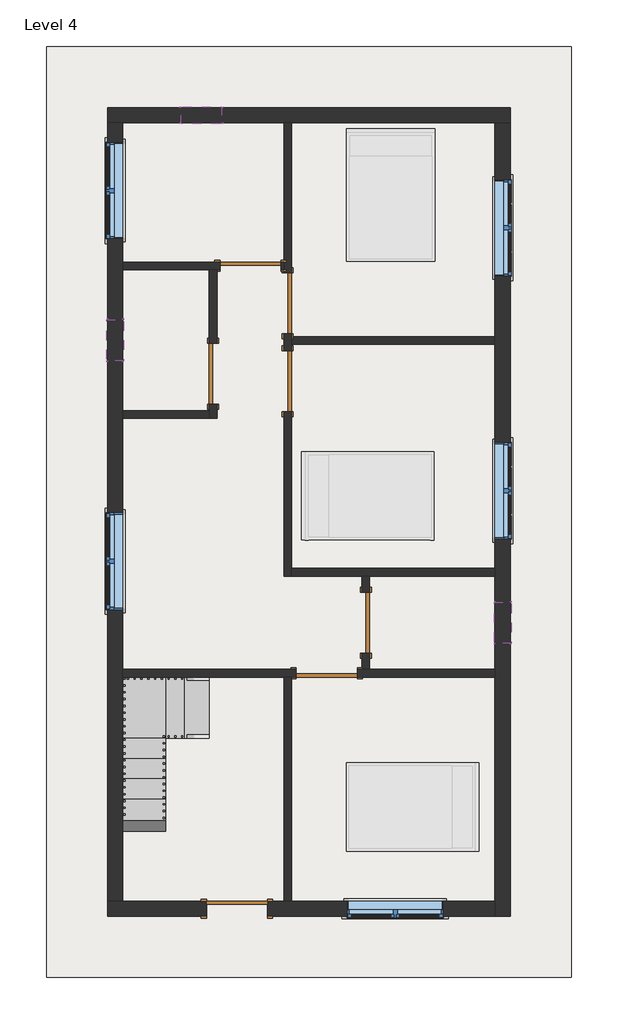
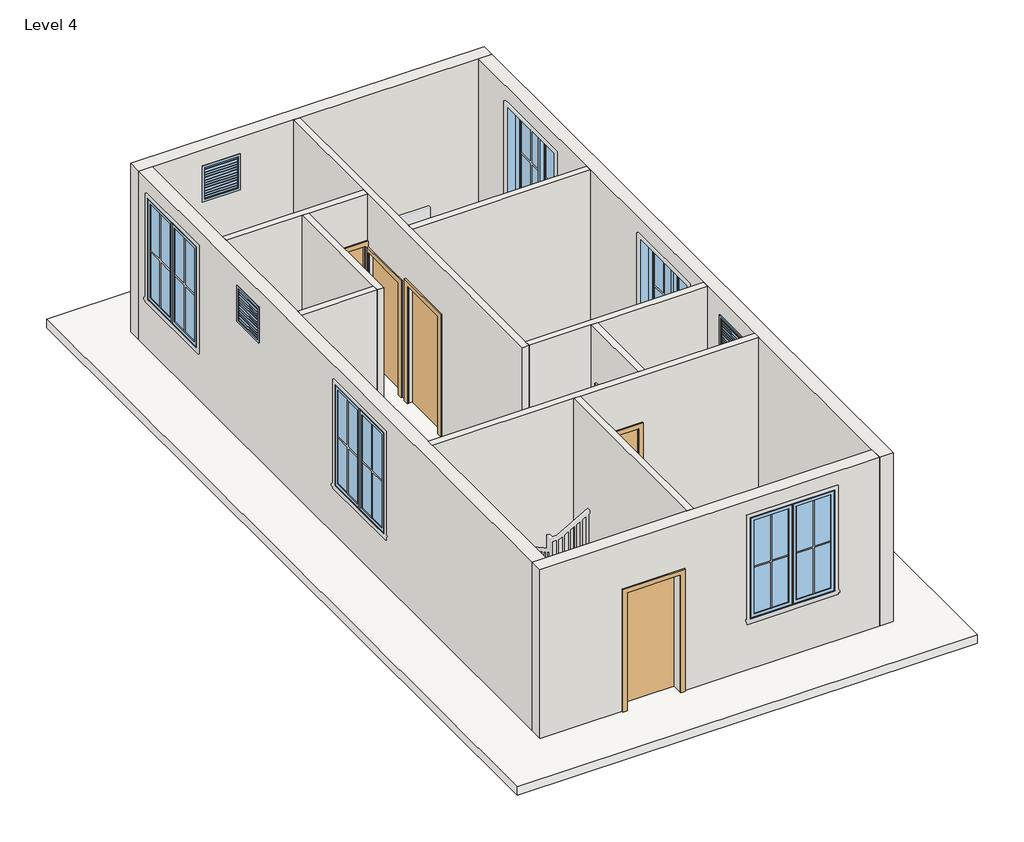
# One storey, part 1 of 2: 13 walls, 8 windows, 7 doors, 1 roof, 1 stair flight.
"""IFC4 building model written with IfcOpenShell, lengths in millimetres."""

from ifc_helpers import new_model, si_unit, frame, origin, place, context, project, spatial, polyline, outline, extrude, faceted_brep, transform, mapped, element, save
from components import door_5e62189b, door_17d80c48, door_e5f9f3c4, door_305aa2a5, door_0ca8825f, window_9ac97e1a, window_f2d8fef0

model = new_model("IFC4")

# Units and contexts
model_context = context("Model", 3, world=origin())
ifc_project = project(units=[si_unit("LENGTHUNIT", "METRE", prefix="MILLI")], contexts=[model_context])

# Site, building, storey
site = spatial("IfcSite", under=ifc_project)
building = spatial("IfcBuilding", under=site)
storey = spatial("IfcBuildingStorey", under=building, Name="Level 4", Elevation=6400.8)

# Doors
placement = place(None, origin())
door_shape = door_5e62189b(model_context)
element("IfcDoor", 1, ObjectType="Single-Flush : 36\" x 80\"", at=placement, inside=storey, context=model_context, shape_type="MappedRepresentation", body=[
    mapped(door_shape, transform((-2690.3389285, 2204.6069249, 6400.8), x_axis=(0.0, -1.0, 0.0), y_axis=(1.0, 0.0, 0.0), z_axis=(0.0, 0.0, 1.0))),
])
element("IfcDoor", 2, ObjectType="Single-Flush : 36\" x 80\"", at=placement, inside=storey, context=model_context, shape_type="MappedRepresentation", body=[
    mapped(door_shape, transform((-404.3389285, -1522.8430751, 6400.8), x_axis=(0.0, 1.0, 0.0), y_axis=(-1.0, 0.0, 0.0), z_axis=(0.0, 0.0, 1.0))),
])
door_2_shape = door_17d80c48(model_context)
element("IfcDoor", 3, ObjectType="Single-Flush : 36\" x 80\"", at=placement, inside=storey, context=model_context, shape_type="MappedRepresentation", body=[
    mapped(door_2_shape, transform((-1572.7389285, 3258.7069249, 6400.8), x_axis=(0.0, -1.0, 0.0), y_axis=(1.0, 0.0, 0.0), z_axis=(0.0, 0.0, 1.0))),
])
door_3_shape = door_e5f9f3c4(model_context)
element("IfcDoor", 4, ObjectType="Single-Flush : 36\" x 84\"", at=placement, inside=storey, context=model_context, shape_type="MappedRepresentation", body=[
    mapped(door_3_shape, transform((-2131.5389285, 3817.5069249, 6400.8), x_axis=(1.0, 0.0, 0.0), y_axis=(0.0, 1.0, 0.0), z_axis=(0.0, 0.0, 1.0))),
])
element("IfcDoor", 5, ObjectType="Single-Flush : 36\" x 84\"", at=placement, inside=storey, context=model_context, shape_type="MappedRepresentation", body=[
    mapped(door_3_shape, transform((-988.5389285, -2278.4930751, 6400.8), x_axis=(-1.0, 0.0, 0.0), y_axis=(0.0, -1.0, 0.0), z_axis=(0.0, 0.0, 1.0))),
])
door_4_shape = door_305aa2a5(model_context)
element("IfcDoor", 6, ObjectType="Single-Flush : 36\" x 84\"", at=placement, inside=storey, context=model_context, shape_type="MappedRepresentation", body=[
    mapped(door_4_shape, transform((-1572.7389285, 2090.3069249, 6400.8), x_axis=(0.0, 1.0, 0.0), y_axis=(-1.0, 0.0, 0.0), z_axis=(0.0, 0.0, 1.0))),
])
door_5_shape = door_0ca8825f(model_context)
element("IfcDoor", 7, ObjectType="Single-Flush : 36\" x 84\"", at=placement, inside=storey, context=model_context, shape_type="MappedRepresentation", body=[
    mapped(door_5_shape, transform((-2334.7389285, -5802.7430751, 6400.8), x_axis=(1.0, 0.0, 0.0), y_axis=(0.0, 1.0, 0.0), z_axis=(0.0, 0.0, 1.0))),
])

# Roof
element("IfcRoof", 8, ObjectType="ROOF 6\"", at=placement, inside=storey, context=model_context, shape_type="SweptSolid", body=[
    extrude(outline(polyline([(-5185.8889285, 7100.4569249), (2675.4110715, 7100.4569249), (2675.4110715, -6831.4430751), (-5185.8889285, -6831.4430751), (-5185.8889285, 7100.4569249)])), frame((0.0, 0.0, 6248.4), z_axis=(0.0, 0.0, 1.0), x_axis=(1.0, 0.0, 0.0)), (0.0, 0.0, 1.0), 152.4),
])

# Stair flight
element("IfcStairFlight", 9, ObjectType="3/4\" Nosing", at=placement, inside=storey, context=model_context, shape_type="Brep", body=[
    faceted_brep([(-2747.4889285, -3250.0430751, 6570.1333333), (-2747.4889285, -2335.6430751, 6570.1333333), (-3128.4889285, -2335.6430751, 6570.1333333), (-3128.4889285, -3250.0430751, 6570.1333333), (-3128.4889285, -3250.0430751, 6506.6333333), (-2754.6326785, -3250.0430751, 6506.6333333), (-2754.6326785, -2335.6430751, 6506.6333333), (-3128.4889285, -2335.6430751, 6506.6333333)], [[[0, 1, 2, 3]], [[0, 3, 4, 5]], [[2, 1, 6, 7]], [[1, 0, 5, 6]], [[4, 7, 6, 5]], [[7, 4, 3, 2]]]),
    faceted_brep([(-3128.4889285, -3250.0430751, 6739.4666667), (-3128.4889285, -2335.6430751, 6739.4666667), (-3401.5389285, -2335.6430751, 6739.4666667), (-3401.5389285, -3250.0430751, 6739.4666667), (-3401.5389285, -3250.0430751, 6675.9666667), (-3135.6326785, -3250.0430751, 6675.9666667), (-3135.6326785, -2335.6430751, 6675.9666667), (-3401.5389285, -2335.6430751, 6675.9666667)], [[[0, 1, 2, 3]], [[0, 3, 4, 5]], [[2, 1, 6, 7]], [[1, 0, 5, 6]], [[4, 7, 6, 5]], [[7, 4, 3, 2]]]),
    faceted_brep([(-3401.5389285, -3269.0930751, 6908.8), (-3401.5389285, -3250.0430751, 6908.8), (-3401.5389285, -2335.6430751, 6908.8), (-4042.8889285, -2335.6430751, 6908.8), (-4042.8889285, -3269.0930751, 6908.8), (-3401.5389285, -3269.0930751, 6845.3), (-3401.5389285, -3250.0430751, 6845.3), (-3408.6826785, -3250.0430751, 6845.3), (-3408.6826785, -2335.6430751, 6845.3), (-4042.8889285, -2335.6430751, 6845.3), (-4042.8889285, -3269.0930751, 6845.3), (-3401.5389285, -3250.0430751, 7078.1333333), (-4042.8889285, -3250.0430751, 7078.1333333), (-4042.8889285, -3285.5502386, 7078.1333333), (-4042.8889285, -3573.8930751, 7078.1333333), (-3401.5389285, -3573.8930751, 7078.1333333), (-3401.5389285, -3285.5502386, 7078.1333333), (-3401.5389285, -3573.8930751, 7005.5200976), (-3401.5389285, -3285.5502386, 6845.3), (-4042.8889285, -3285.5502386, 6845.3), (-4042.8889285, -3573.8930751, 7005.5200976), (-3401.5389285, -3554.8430751, 7247.4666667), (-4042.8889285, -3554.8430751, 7247.4666667), (-4042.8889285, -3878.6930751, 7247.4666667), (-3401.5389285, -3878.6930751, 7247.4666667), (-3401.5389285, -3878.6930751, 7174.8847552), (-4042.8889285, -3878.6930751, 7174.8847552), (-3401.5389285, -3859.6430751, 7416.8), (-4042.8889285, -3859.6430751, 7416.8), (-4042.8889285, -4183.4930751, 7416.8), (-3401.5389285, -4183.4930751, 7416.8), (-3401.5389285, -4183.4930751, 7344.2494128), (-4042.8889285, -4183.4930751, 7344.2494128), (-3401.5389285, -4164.4430751, 7586.1333333), (-4042.8889285, -4164.4430751, 7586.1333333), (-4042.8889285, -4488.2930751, 7586.1333333), (-3401.5389285, -4488.2930751, 7586.1333333), (-3401.5389285, -4488.2930751, 7513.6140703), (-4042.8889285, -4488.2930751, 7513.6140703), (-3401.5389285, -4792.8112092, 7755.4666667), (-3401.5389285, -4469.2430751, 7755.4666667), (-4042.8889285, -4469.2430751, 7755.4666667), (-4042.8889285, -4792.8112092, 7755.4666667), (-3401.5389285, -4773.7612092, 7924.8), (-3401.5389285, -5114.0119996, 7924.8), (-3401.5389285, -5114.0119996, 7861.3), (-4042.8889285, -4792.8112092, 7682.8221068), (-4042.8889285, -4773.7612092, 7924.8), (-4042.8889285, -5114.0119996, 7924.8), (-4042.8889285, -5688.4430751, 7924.8), (-3401.5389285, -5688.4430751, 7924.8), (-4042.8889285, -5114.0119996, 7861.3), (-4042.8889285, -5688.4430751, 7861.3), (-3401.5389285, -5688.4430751, 7861.3)], [[[0, 1, 2, 3, 4]], [[1, 0, 5, 6]], [[7, 1, 6]], [[3, 2, 8, 9]], [[4, 3, 9, 10]], [[11, 12, 13, 14, 15, 16]], [[0, 11, 16, 15, 17, 18, 5]], [[12, 4, 10, 19, 20, 14, 13]], [[21, 22, 23, 24]], [[21, 24, 25, 17, 15]], [[23, 22, 14, 20, 26]], [[27, 28, 29, 30]], [[27, 30, 31, 25, 24]], [[29, 28, 23, 26, 32]], [[33, 34, 35, 36]], [[33, 36, 37, 31, 30]], [[35, 34, 29, 32, 38]], [[39, 40, 41, 42]], [[39, 43, 44, 45, 37, 36, 40]], [[42, 41, 35, 38, 46]], [[43, 47, 48, 49, 50, 44]], [[47, 42, 46, 51, 52, 49, 48]], [[50, 49, 52, 53]], [[2, 1, 7, 8]], [[0, 4, 12, 11]], [[15, 14, 22, 21]], [[24, 23, 28, 27]], [[30, 29, 34, 33]], [[36, 35, 41, 40]], [[39, 42, 47, 43]], [[18, 19, 10, 9, 8, 7, 6, 5]], [[19, 18, 17, 25, 31, 37, 45, 51, 46, 38, 32, 26, 20]], [[45, 53, 52, 51]], [[53, 45, 44, 50]]]),
    faceted_brep([(-3401.5389285, -4773.7612092, 8094.1333333), (-3401.5389285, -5688.4430751, 8094.1333333), (-3128.4889285, -5688.4430751, 8094.1333333), (-3128.4889285, -4773.7612092, 8094.1333333), (-3394.3951785, -4773.7612092, 8030.6333333), (-3128.4889285, -4773.7612092, 8030.6333333), (-3394.3951785, -5688.4430751, 8030.6333333), (-3128.4889285, -5688.4430751, 8030.6333333)], [[[0, 1, 2, 3]], [[4, 0, 3, 5]], [[2, 1, 6, 7]], [[1, 0, 4, 6]], [[5, 7, 6, 4]], [[7, 5, 3, 2]]]),
    faceted_brep([(-3128.4889285, -4773.7612092, 8263.4666667), (-3128.4889285, -5688.4430751, 8263.4666667), (-2793.6303845, -5688.4430751, 8263.4666667), (-2793.6303845, -4773.7612092, 8263.4666667), (-2793.6303845, -4773.7612092, 8199.9666667), (-3121.3451785, -4773.7612092, 8199.9666667), (-3121.3451785, -5688.4430751, 8199.9666667), (-2793.6303845, -5688.4430751, 8199.9666667)], [[[0, 1, 2, 3]], [[0, 3, 4, 5]], [[2, 1, 6, 7]], [[3, 2, 7, 4]], [[1, 0, 5, 6]], [[6, 5, 4, 7]]]),
])

# Walls
element("IfcWall", 10, ObjectType="WALL 4.5\"", at=placement, inside=storey, context=model_context, shape_type="Brep", body=[
    faceted_brep([(-1629.8889285, 2801.5069249, 8432.8), (-1629.8889285, 2801.5069249, 6400.8), (-1629.8889285, 2547.5069249, 6400.8), (-1629.8889285, 2547.5069249, 8534.4), (-1629.8889285, 1633.1069249, 8534.4), (-1629.8889285, 1633.1069249, 6400.8), (-1629.8889285, -824.3430751, 6400.8), (-1629.8889285, -824.3430751, 9448.8), (-1629.8889285, 3760.3569249, 9448.8), (-1629.8889285, 3874.6569249, 9448.8), (-1629.8889285, 5957.4569249, 9448.8), (-1629.8889285, 5957.4569249, 6400.8), (-1629.8889285, 3874.6569249, 6400.8), (-1629.8889285, 3760.3569249, 6400.8), (-1629.8889285, 3715.9069249, 6400.8), (-1629.8889285, 3715.9069249, 8432.8), (-1515.5889285, 2547.5069249, 6400.8), (-1515.5889285, 2642.7569249, 6400.8), (-1515.5889285, 2757.0569249, 6400.8), (-1515.5889285, 2801.5069249, 6400.8), (-1515.5889285, 2801.5069249, 8432.8), (-1515.5889285, 3715.9069249, 8432.8), (-1515.5889285, 3715.9069249, 6400.8), (-1515.5889285, 5957.4569249, 6400.8), (-1515.5889285, 5957.4569249, 9448.8), (-1515.5889285, 2757.0569249, 9448.8), (-1515.5889285, 2642.7569249, 9448.8), (-1515.5889285, -710.0430751, 9448.8), (-1515.5889285, -824.3430751, 9448.8), (-1515.5889285, -824.3430751, 6400.8), (-1515.5889285, -710.0430751, 6400.8), (-1515.5889285, 1633.1069249, 6400.8), (-1515.5889285, 1633.1069249, 8534.4), (-1515.5889285, 2547.5069249, 8534.4)], [[[0, 1, 2, 3, 4, 5, 6, 7, 8, 9, 10, 11, 12, 13, 14, 15]], [[16, 17, 18, 19, 20, 21, 22, 23, 24, 25, 26, 27, 28, 29, 30, 31, 32, 33]], [[31, 30, 29, 6, 5]], [[2, 1, 19, 18, 17, 16]], [[14, 13, 12, 11, 23, 22]], [[11, 10, 24, 23]], [[3, 2, 16, 33]], [[4, 3, 33, 32]], [[5, 4, 32, 31]], [[20, 19, 1, 0]], [[21, 20, 0, 15]], [[22, 21, 15, 14]], [[10, 9, 8, 7, 28, 27, 26, 25, 24]], [[7, 6, 29, 28]]]),
])
element("IfcWall", 11, ObjectType="WALL 4.5\"", at=placement, inside=storey, context=model_context, shape_type="Brep", body=[
    faceted_brep([(1532.4110715, -710.0430751, 6400.8), (-1515.5889285, -710.0430751, 6400.8), (-1515.5889285, -710.0430751, 9448.8), (1532.4110715, -710.0430751, 9448.8), (1532.4110715, -824.3430751, 6400.8), (1532.4110715, -824.3430751, 9448.8), (-347.1889285, -824.3430751, 9448.8), (-461.4889285, -824.3430751, 9448.8), (-1515.5889285, -824.3430751, 9448.8), (-1515.5889285, -824.3430751, 6400.8), (-461.4889285, -824.3430751, 6400.8), (-347.1889285, -824.3430751, 6400.8)], [[[0, 1, 2, 3]], [[4, 5, 6, 7, 8, 9, 10, 11]], [[1, 0, 4, 11, 10, 9]], [[0, 3, 5, 4]], [[3, 2, 8, 7, 6, 5]], [[2, 1, 9, 8]]]),
])
element("IfcWall", 12, ObjectType="WALL 4.5\"", at=placement, inside=storey, context=model_context, shape_type="SweptSolid", body=[
    extrude(outline(polyline([(-1515.5889285, 2757.0569249), (1532.4110715, 2757.0569249), (1532.4110715, 2642.7569249), (-1515.5889285, 2642.7569249), (-1515.5889285, 2757.0569249)])), frame((0.0, 0.0, 6400.8), z_axis=(0.0, 0.0, 1.0), x_axis=(1.0, 0.0, 0.0)), (0.0, 0.0, 1.0), 3048.0),
])
element("IfcWall", 13, ObjectType="WALL 4.5\"", at=placement, inside=storey, context=model_context, shape_type="Brep", body=[
    faceted_brep([(-1674.3389285, 3760.3569249, 8534.4), (-1674.3389285, 3760.3569249, 6400.8), (-1629.8889285, 3760.3569249, 6400.8), (-1629.8889285, 3760.3569249, 9448.8), (-2633.1889285, 3760.3569249, 9448.8), (-2747.4889285, 3760.3569249, 9448.8), (-4042.8889285, 3760.3569249, 9448.8), (-4042.8889285, 3760.3569249, 6400.8), (-2747.4889285, 3760.3569249, 6400.8), (-2633.1889285, 3760.3569249, 6400.8), (-2588.7389285, 3760.3569249, 6400.8), (-2588.7389285, 3760.3569249, 8534.4), (-1629.8889285, 3874.6569249, 6400.8), (-1674.3389285, 3874.6569249, 6400.8), (-1674.3389285, 3874.6569249, 8534.4), (-2588.7389285, 3874.6569249, 8534.4), (-2588.7389285, 3874.6569249, 6400.8), (-4042.8889285, 3874.6569249, 6400.8), (-4042.8889285, 3874.6569249, 9448.8), (-1629.8889285, 3874.6569249, 9448.8)], [[[0, 1, 2, 3, 4, 5, 6, 7, 8, 9, 10, 11]], [[12, 13, 14, 15, 16, 17, 18, 19]], [[2, 1, 13, 12]], [[10, 9, 8, 7, 17, 16]], [[7, 6, 18, 17]], [[3, 2, 12, 19]], [[14, 13, 1, 0]], [[15, 14, 0, 11]], [[16, 15, 11, 10]], [[6, 5, 4, 3, 19, 18]]]),
])
element("IfcWall", 14, ObjectType="WALL 4.5\"", at=placement, inside=storey, context=model_context, shape_type="Brep", body=[
    faceted_brep([(-2747.4889285, 1747.4069249, 8432.8), (-2747.4889285, 1747.4069249, 6400.8), (-2747.4889285, 1652.1569249, 6400.8), (-2747.4889285, 1537.8569249, 6400.8), (-2747.4889285, 1537.8569249, 9448.8), (-2747.4889285, 1652.1569249, 9448.8), (-2747.4889285, 3760.3569249, 9448.8), (-2747.4889285, 3760.3569249, 6400.8), (-2747.4889285, 2661.8069249, 6400.8), (-2747.4889285, 2661.8069249, 8432.8), (-2633.1889285, 1537.8569249, 6400.8), (-2633.1889285, 1747.4069249, 6400.8), (-2633.1889285, 1747.4069249, 8432.8), (-2633.1889285, 2661.8069249, 8432.8), (-2633.1889285, 2661.8069249, 6400.8), (-2633.1889285, 3760.3569249, 6400.8), (-2633.1889285, 3760.3569249, 9448.8), (-2633.1889285, 1537.8569249, 9448.8)], [[[0, 1, 2, 3, 4, 5, 6, 7, 8, 9]], [[10, 11, 12, 13, 14, 15, 16, 17]], [[8, 7, 15, 14]], [[3, 2, 1, 11, 10]], [[7, 6, 16, 15]], [[4, 3, 10, 17]], [[12, 11, 1, 0]], [[13, 12, 0, 9]], [[14, 13, 9, 8]], [[6, 5, 4, 17, 16]]]),
])
element("IfcWall", 15, ObjectType="WALL 4.5\"", at=placement, inside=storey, context=model_context, shape_type="SweptSolid", body=[
    extrude(outline(polyline([(-4042.8889285, 1652.1569249), (-2747.4889285, 1652.1569249), (-2747.4889285, 1537.8569249), (-4042.8889285, 1537.8569249), (-4042.8889285, 1652.1569249)])), frame((0.0, 0.0, 6400.8), z_axis=(0.0, 0.0, 1.0), x_axis=(1.0, 0.0, 0.0)), (0.0, 0.0, 1.0), 3048.0),
])
element("IfcWall", 16, ObjectType="WALL 4.5\"", at=placement, inside=storey, context=model_context, shape_type="Brep", body=[
    faceted_brep([(-4042.8889285, -2335.6430751, 6400.8), (-1629.8889285, -2335.6430751, 6400.8), (-1515.5889285, -2335.6430751, 6400.8), (-1445.7389285, -2335.6430751, 6400.8), (-1445.7389285, -2335.6430751, 8534.4), (-531.3389285, -2335.6430751, 8534.4), (-531.3389285, -2335.6430751, 6400.8), (1532.4110715, -2335.6430751, 6400.8), (1532.4110715, -2335.6430751, 9448.8), (-1515.5889285, -2335.6430751, 9448.8), (-1629.8889285, -2335.6430751, 9448.8), (-4042.8889285, -2335.6430751, 9448.8), (-1445.7389285, -2221.3430751, 8534.4), (-1445.7389285, -2221.3430751, 6400.8), (-4042.8889285, -2221.3430751, 6400.8), (-4042.8889285, -2221.3430751, 9448.8), (-461.4889285, -2221.3430751, 9448.8), (-347.1889285, -2221.3430751, 9448.8), (1532.4110715, -2221.3430751, 9448.8), (1532.4110715, -2221.3430751, 6400.8), (-347.1889285, -2221.3430751, 6400.8), (-461.4889285, -2221.3430751, 6400.8), (-531.3389285, -2221.3430751, 6400.8), (-531.3389285, -2221.3430751, 8534.4)], [[[0, 1, 2, 3, 4, 5, 6, 7, 8, 9, 10, 11]], [[12, 13, 14, 15, 16, 17, 18, 19, 20, 21, 22, 23]], [[14, 13, 3, 2, 1, 0]], [[22, 21, 20, 19, 7, 6]], [[8, 7, 19, 18]], [[0, 11, 15, 14]], [[4, 3, 13, 12]], [[5, 4, 12, 23]], [[6, 5, 23, 22]], [[11, 10, 9, 8, 18, 17, 16, 15]]]),
])
element("IfcWall", 17, ObjectType="WALL 4.5\"", at=placement, inside=storey, context=model_context, shape_type="SweptSolid", body=[
    extrude(outline(polyline([(-824.3430751, 6400.8), (-1065.6430751, 6400.8), (-1065.6430751, 8432.8), (-1980.0430751, 8432.8), (-1980.0430751, 6400.8), (-2221.3430751, 6400.8), (-2221.3430751, 9448.8), (-824.3430751, 9448.8), (-824.3430751, 6400.8)])), frame((-461.4889285, 0.0, 0.0), z_axis=(1.0, 0.0, 0.0), x_axis=(0.0, 1.0, 0.0)), (0.0, 0.0, 1.0), 114.3),
])
element("IfcWall", 18, ObjectType="WALL 4.5\"", at=placement, inside=storey, context=model_context, shape_type="SweptSolid", body=[
    extrude(outline(polyline([(-1629.8889285, -5688.4430751), (-1629.8889285, -2335.6430751), (-1515.5889285, -2335.6430751), (-1515.5889285, -5688.4430751), (-1629.8889285, -5688.4430751)])), frame((0.0, 0.0, 6400.8), z_axis=(0.0, 0.0, 1.0), x_axis=(1.0, 0.0, 0.0)), (0.0, 0.0, 1.0), 3048.0),
])
element("IfcWall", 19, ObjectType="WALL 9\"", at=placement, inside=storey, context=model_context, shape_type="Brep", body=[
    faceted_brep([(-4271.4889285, 5957.4569249, 6400.8), (-4042.8889285, 5957.4569249, 6400.8), (-1629.8889285, 5957.4569249, 6400.8), (-1515.5889285, 5957.4569249, 6400.8), (1532.4110715, 5957.4569249, 6400.8), (1761.0110715, 5957.4569249, 6400.8), (1761.0110715, 5957.4569249, 9448.8), (1532.4110715, 5957.4569249, 9448.8), (-1515.5889285, 5957.4569249, 9448.8), (-1629.8889285, 5957.4569249, 9448.8), (-4042.8889285, 5957.4569249, 9448.8), (-4271.4889285, 5957.4569249, 9448.8), (-2560.1639285, 5957.4569249, 9144.0), (-2560.1639285, 5957.4569249, 8534.4), (-3169.7639285, 5957.4569249, 8534.4), (-3169.7639285, 5957.4569249, 9144.0), (-4271.4889285, 6186.0569249, 6400.8), (-4271.4889285, 6186.0569249, 9448.8), (1761.0110715, 6186.0569249, 9448.8), (1761.0110715, 6186.0569249, 6400.8), (-2560.1639285, 6186.0569249, 9144.0), (-3169.7639285, 6186.0569249, 9144.0), (-3169.7639285, 6186.0569249, 8534.4), (-2560.1639285, 6186.0569249, 8534.4)], [[[0, 1, 2, 3, 4, 5, 6, 7, 8, 9, 10, 11], [12, 13, 14, 15]], [[16, 17, 18, 19], [20, 21, 22, 23]], [[5, 4, 3, 2, 1, 0, 16, 19]], [[6, 5, 19, 18]], [[0, 11, 17, 16]], [[13, 12, 20, 23]], [[14, 13, 23, 22]], [[15, 14, 22, 21]], [[12, 15, 21, 20]], [[11, 10, 9, 8, 7, 6, 18, 17]]]),
])
element("IfcWall", 20, ObjectType="WALL 9\"", at=placement, inside=storey, context=model_context, shape_type="Brep", body=[
    faceted_brep([(1532.4110715, 5957.4569249, 6400.8), (1532.4110715, 2757.0569249, 6400.8), (1532.4110715, 2642.7569249, 6400.8), (1532.4110715, -710.0430751, 6400.8), (1532.4110715, -824.3430751, 6400.8), (1532.4110715, -2221.3430751, 6400.8), (1532.4110715, -2335.6430751, 6400.8), (1532.4110715, -5688.4430751, 6400.8), (1532.4110715, -5917.0430751, 6400.8), (1532.4110715, -5917.0430751, 9448.8), (1532.4110715, -5688.4430751, 9448.8), (1532.4110715, -2335.6430751, 9448.8), (1532.4110715, -2221.3430751, 9448.8), (1532.4110715, -824.3430751, 9448.8), (1532.4110715, -710.0430751, 9448.8), (1532.4110715, 2642.7569249, 9448.8), (1532.4110715, 2757.0569249, 9448.8), (1532.4110715, 5957.4569249, 9448.8), (1532.4110715, 3661.9319249, 9144.0), (1532.4110715, 3661.9319249, 7315.2), (1532.4110715, 5109.7319249, 7315.2), (1532.4110715, 5109.7319249, 9144.0), (1532.4110715, -271.8930751, 9144.0), (1532.4110715, -271.8930751, 7315.2), (1532.4110715, 1175.9069249, 7315.2), (1532.4110715, 1175.9069249, 9144.0), (1532.4110715, -1827.6430751, 9144.0), (1532.4110715, -1827.6430751, 8534.4), (1532.4110715, -1218.0430751, 8534.4), (1532.4110715, -1218.0430751, 9144.0), (1761.0110715, 5957.4569249, 6400.8), (1761.0110715, 5957.4569249, 9448.8), (1761.0110715, -5917.0430751, 9448.8), (1761.0110715, -5917.0430751, 6400.8), (1761.0110715, 3661.9319249, 9144.0), (1761.0110715, 5109.7319249, 9144.0), (1761.0110715, 5109.7319249, 7315.2), (1761.0110715, 3661.9319249, 7315.2), (1761.0110715, -271.8930751, 9144.0), (1761.0110715, 1175.9069249, 9144.0), (1761.0110715, 1175.9069249, 7315.2), (1761.0110715, -271.8930751, 7315.2), (1761.0110715, -1827.6430751, 9144.0), (1761.0110715, -1218.0430751, 9144.0), (1761.0110715, -1218.0430751, 8534.4), (1761.0110715, -1827.6430751, 8534.4)], [[[0, 1, 2, 3, 4, 5, 6, 7, 8, 9, 10, 11, 12, 13, 14, 15, 16, 17], [18, 19, 20, 21], [22, 23, 24, 25], [26, 27, 28, 29]], [[30, 31, 32, 33], [34, 35, 36, 37], [38, 39, 40, 41], [42, 43, 44, 45]], [[8, 7, 6, 5, 4, 3, 2, 1, 0, 30, 33]], [[0, 17, 31, 30]], [[9, 8, 33, 32]], [[19, 18, 34, 37]], [[20, 19, 37, 36]], [[21, 20, 36, 35]], [[18, 21, 35, 34]], [[23, 22, 38, 41]], [[24, 23, 41, 40]], [[25, 24, 40, 39]], [[22, 25, 39, 38]], [[27, 26, 42, 45]], [[28, 27, 45, 44]], [[29, 28, 44, 43]], [[26, 29, 43, 42]], [[17, 16, 15, 14, 13, 12, 11, 10, 9, 32, 31]]]),
])
element("IfcWall", 21, ObjectType="WALL 9\"", at=placement, inside=storey, context=model_context, shape_type="Brep", body=[
    faceted_brep([(1532.4110715, -5688.4430751, 6400.8), (-1515.5889285, -5688.4430751, 6400.8), (-1629.8889285, -5688.4430751, 6400.8), (-1877.5389285, -5688.4430751, 6400.8), (-1877.5389285, -5688.4430751, 8534.4), (-2791.9389285, -5688.4430751, 8534.4), (-2791.9389285, -5688.4430751, 6400.8), (-4042.8889285, -5688.4430751, 6400.8), (-4271.4889285, -5688.4430751, 6400.8), (-4271.4889285, -5688.4430751, 9448.8), (-4042.8889285, -5688.4430751, 9448.8), (-1629.8889285, -5688.4430751, 9448.8), (-1515.5889285, -5688.4430751, 9448.8), (1532.4110715, -5688.4430751, 9448.8), (-686.9139285, -5688.4430751, 9144.0), (-686.9139285, -5688.4430751, 7315.2), (760.8860715, -5688.4430751, 7315.2), (760.8860715, -5688.4430751, 9144.0), (-1877.5389285, -5917.0430751, 8534.4), (-1877.5389285, -5917.0430751, 6400.8), (1532.4110715, -5917.0430751, 6400.8), (1532.4110715, -5917.0430751, 9448.8), (-4271.4889285, -5917.0430751, 9448.8), (-4271.4889285, -5917.0430751, 6400.8), (-2791.9389285, -5917.0430751, 6400.8), (-2791.9389285, -5917.0430751, 8534.4), (-686.9139285, -5917.0430751, 9144.0), (760.8860715, -5917.0430751, 9144.0), (760.8860715, -5917.0430751, 7315.2), (-686.9139285, -5917.0430751, 7315.2)], [[[0, 1, 2, 3, 4, 5, 6, 7, 8, 9, 10, 11, 12, 13], [14, 15, 16, 17]], [[18, 19, 20, 21, 22, 23, 24, 25], [26, 27, 28, 29]], [[24, 23, 8, 7, 6]], [[20, 19, 3, 2, 1, 0]], [[0, 13, 21, 20]], [[9, 8, 23, 22]], [[15, 14, 26, 29]], [[16, 15, 29, 28]], [[17, 16, 28, 27]], [[14, 17, 27, 26]], [[4, 3, 19, 18]], [[5, 4, 18, 25]], [[6, 5, 25, 24]], [[13, 12, 11, 10, 9, 22, 21]]]),
])
element("IfcWall", 22, ObjectType="WALL 9\"", at=placement, inside=storey, context=model_context, shape_type="Brep", body=[
    faceted_brep([(-4042.8889285, -5688.4430751, 6400.8), (-4042.8889285, -2335.6430751, 6400.8), (-4042.8889285, -2221.3430751, 6400.8), (-4042.8889285, 1537.8569249, 6400.8), (-4042.8889285, 1652.1569249, 6400.8), (-4042.8889285, 3760.3569249, 6400.8), (-4042.8889285, 3874.6569249, 6400.8), (-4042.8889285, 5957.4569249, 6400.8), (-4042.8889285, 5957.4569249, 9448.8), (-4042.8889285, 3874.6569249, 9448.8), (-4042.8889285, 3760.3569249, 9448.8), (-4042.8889285, 1652.1569249, 9448.8), (-4042.8889285, 1537.8569249, 9448.8), (-4042.8889285, -2221.3430751, 9448.8), (-4042.8889285, -2335.6430751, 9448.8), (-4042.8889285, -5688.4430751, 9448.8), (-4042.8889285, 5668.5319249, 9144.0), (-4042.8889285, 5668.5319249, 7315.2), (-4042.8889285, 4220.7319249, 7315.2), (-4042.8889285, 4220.7319249, 9144.0), (-4042.8889285, 121.8069249, 9144.0), (-4042.8889285, 121.8069249, 7315.2), (-4042.8889285, -1325.9930751, 7315.2), (-4042.8889285, -1325.9930751, 9144.0), (-4042.8889285, 2401.4569249, 9144.0), (-4042.8889285, 3011.0569249, 9144.0), (-4042.8889285, 3011.0569249, 8534.4), (-4042.8889285, 2401.4569249, 8534.4), (-4271.4889285, -5688.4430751, 6400.8), (-4271.4889285, -5688.4430751, 9448.8), (-4271.4889285, 5957.4569249, 9448.8), (-4271.4889285, 5957.4569249, 6400.8), (-4271.4889285, 5668.5319249, 9144.0), (-4271.4889285, 4220.7319249, 9144.0), (-4271.4889285, 4220.7319249, 7315.2), (-4271.4889285, 5668.5319249, 7315.2), (-4271.4889285, 121.8069249, 9144.0), (-4271.4889285, -1325.9930751, 9144.0), (-4271.4889285, -1325.9930751, 7315.2), (-4271.4889285, 121.8069249, 7315.2), (-4271.4889285, 2401.4569249, 9144.0), (-4271.4889285, 2401.4569249, 8534.4), (-4271.4889285, 3011.0569249, 8534.4), (-4271.4889285, 3011.0569249, 9144.0)], [[[0, 1, 2, 3, 4, 5, 6, 7, 8, 9, 10, 11, 12, 13, 14, 15], [16, 17, 18, 19], [20, 21, 22, 23], [24, 25, 26, 27]], [[28, 29, 30, 31], [32, 33, 34, 35], [36, 37, 38, 39], [40, 41, 42, 43]], [[7, 6, 5, 4, 3, 2, 1, 0, 28, 31]], [[0, 15, 29, 28]], [[8, 7, 31, 30]], [[17, 16, 32, 35]], [[18, 17, 35, 34]], [[19, 18, 34, 33]], [[16, 19, 33, 32]], [[21, 20, 36, 39]], [[22, 21, 39, 38]], [[23, 22, 38, 37]], [[20, 23, 37, 36]], [[41, 40, 24, 27]], [[42, 41, 27, 26]], [[43, 42, 26, 25]], [[40, 43, 25, 24]], [[15, 14, 13, 12, 11, 10, 9, 8, 30, 29]]]),
])

# Windows
window_shape = window_9ac97e1a(model_context)
element("IfcWindow", 23, ObjectType="Window-Casement-Double : 57\" x 72\"", at=placement, inside=storey, context=model_context, shape_type="MappedRepresentation", body=[
    mapped(window_shape, transform((-4157.1889285, 4944.6319249, 6400.8), x_axis=(0.0, 1.0, 0.0), y_axis=(-1.0, 0.0, 0.0), z_axis=(0.0, 0.0, 1.0))),
])
element("IfcWindow", 24, ObjectType="Window-Casement-Double : 57\" x 72\"", at=placement, inside=storey, context=model_context, shape_type="MappedRepresentation", body=[
    mapped(window_shape, transform((1646.7110715, 4385.8319249, 6400.8), x_axis=(0.0, -1.0, 0.0), y_axis=(1.0, 0.0, 0.0), z_axis=(0.0, 0.0, 1.0))),
])
element("IfcWindow", 25, ObjectType="Window-Casement-Double : 57\" x 72\"", at=placement, inside=storey, context=model_context, shape_type="MappedRepresentation", body=[
    mapped(window_shape, transform((-4157.1889285, -602.0930751, 6400.8), x_axis=(0.0, 1.0, 0.0), y_axis=(-1.0, 0.0, 0.0), z_axis=(0.0, 0.0, 1.0))),
])
element("IfcWindow", 26, ObjectType="Window-Casement-Double : 57\" x 72\"", at=placement, inside=storey, context=model_context, shape_type="MappedRepresentation", body=[
    mapped(window_shape, transform((1646.7110715, 452.0069249, 6400.8), x_axis=(0.0, -1.0, 0.0), y_axis=(1.0, 0.0, 0.0), z_axis=(0.0, 0.0, 1.0))),
])
element("IfcWindow", 27, ObjectType="Window-Casement-Double : 57\" x 72\"", at=placement, inside=storey, context=model_context, shape_type="MappedRepresentation", body=[
    mapped(window_shape, transform((36.9860715, -5802.7430751, 6400.8), x_axis=(-1.0, 0.0, 0.0), y_axis=(0.0, -1.0, 0.0), z_axis=(0.0, 0.0, 1.0))),
])
window_2_shape = window_f2d8fef0(model_context)
element("IfcWindow", 28, ObjectType="Window-Louvers : 24\" x 24\"", at=placement, inside=storey, context=model_context, shape_type="MappedRepresentation", body=[
    mapped(window_2_shape, transform((-2864.9639285, 6065.4069249, 7620.0), x_axis=(-1.0, 0.0, 0.0), y_axis=(0.0, -1.0, 0.0), z_axis=(0.0, 0.0, 1.0))),
])
element("IfcWindow", 29, ObjectType="Window-Louvers : 24\" x 24\"", at=placement, inside=storey, context=model_context, shape_type="MappedRepresentation", body=[
    mapped(window_2_shape, transform((-4163.5389285, 2706.2569249, 7620.0), x_axis=(0.0, 1.0, 0.0), y_axis=(-1.0, 0.0, 0.0), z_axis=(0.0, 0.0, 1.0))),
])
element("IfcWindow", 30, ObjectType="Window-Louvers : 24\" x 24\"", at=placement, inside=storey, context=model_context, shape_type="MappedRepresentation", body=[
    mapped(window_2_shape, transform((1640.3610715, -1522.8430751, 7620.0), x_axis=(0.0, 1.0, 0.0), y_axis=(-1.0, 0.0, 0.0), z_axis=(0.0, 0.0, 1.0))),
])

save(model, "model.ifc")

# Revit data of these elements
# Type "Single-Flush : 36\" x 80\""
#   Type Mark = "6"
#   Construction Type Id = "MDOOR"
#   Assembly Code = "C1020"
#   Analytic Construction = "Metal"
#   Thickness = 0' - 2"
#   Heat Transfer Coefficient (U) = 0.651978 BTU/(h·ft²·°F)
#   Height = 6' - 8"
#   Trim Projection Ext = 0' - 1"
#   Trim Projection Int = 0' - 1"
#   Trim Width = 0' - 3"
#   Width = 3' - 0"
#   Define Thermal Properties by = 1
#   Define Thermal Properties by = 1
#   Door Material = Door - Panel
#   Frame Material = Door - Frame
#   Visual Light Transmittance = 0
#   Solar Heat Gain Coefficient = 0
#   Function = (empty or 0)
#   Wall Closure = (empty or 0)
# Type "Single-Flush : 36\" x 84\""
#   Type Mark = "1"
#   Construction Type Id = "MDOOR"
#   Assembly Code = "C1020"
#   Analytic Construction = "Metal"
#   Thickness = 0' - 2"
#   Heat Transfer Coefficient (U) = 0.651978 BTU/(h·ft²·°F)
#   Height = 7' - 0"
#   Trim Projection Ext = 0' - 1"
#   Trim Projection Int = 0' - 1"
#   Trim Width = 0' - 3"
#   Width = 3' - 0"
#   Define Thermal Properties by = 1
#   Define Thermal Properties by = 1
#   Door Material = Door - Panel
#   Frame Material = Door - Frame
#   Visual Light Transmittance = 0
#   Solar Heat Gain Coefficient = 0
#   Function = (empty or 0)
#   Wall Closure = (empty or 0)
# Type "ROOF 6\""
#   Assembly Code = "B1020"
#   Layers, outside or top first: 0' - 6" no material (function 1)
# Type "WALL 4.5\""
#   Assembly Code = "B2010"
#   Layers, outside or top first: 0' - 4 1/2" no material (function 1)
# Type "WALL 9\""
#   Assembly Code = "B2010"
#   Layers, outside or top first: 0' - 9" no material (function 1)
# Type "Window-Casement-Double : 57\" x 72\""
#   Type Mark = "17"
#   Fire Rating = "0.5h"
#   Assembly Code = "B2020100"
#   Analytic Construction = "Double glazing - domestic"
#   Frame Extension [instance default] = 0' - 0 1/4"
#   Window Inset [instance default] = 0' - 0"
#   Wall Thickness [instance default] = 0' - 6"
#   Interior Wall Closure [instance default] = 0' - 2 1/4"
#   Half Width = 2' - 4 1/2"
#   Visual Light Transmittance = 0.81
#   Thermal Resistance (R) = 1.8146 (h·ft²·°F)/BTU
#   Solar Heat Gain Coefficient = 0.76
#   Rough Width = 4' - 9 1/2"
#   Rough Height = 6' - 0 1/2"
#   Height = 6' - 0"
#   Heat Transfer Coefficient (U) = 0.5511 BTU/(h·ft²·°F)
#   Exterior Wall Closure [instance default] = 0' - 1 1/4"
#   Extension Jamb [instance default] = 0' - 2 1/4"
#   Default Sill Height = 3' - 0"
#   Width = 4' - 9"
#   Define Thermal Properties by = 0
#   Muntin Visibility = yes
#   Interior Trim Visibility [instance default] = yes
#   Exterior Trim Visibility [instance default] = yes
#   Extension Jamb Visibility [instance default] = yes
#   Interior Trim Material = Wood - Stained
#   Muntin Pattern = Muntin Pattern_2x2 : Muntin Pattern_2x2
#   Interior Trim = Trim-Window-Interior-Flat : Picture Frame
#   Interior Frame Material = Wood - Stained
#   Glass Panel Material = Glass
#   Exterior Trim Material = Clad - White
#   Exterior Trim = Trim-Window-Exterior-Flat : with Sill
#   Exterior Frame Material = Clad - White
#   Wall Closure = (empty or 0)
# Type "Window-Louvers : 24\" x 24\""
#   Type Mark = "18"
#   Construction Type Id = "GSP4R"
#   Assembly Code = "B20"
#   Analytic Construction = "1/8 in Pilkington single glazing"
#   Visual Light Transmittance = 0.9
#   Thermal Resistance (R) = 1.53941 (h·ft²·°F)/BTU
#   Solar Heat Gain Coefficient = 0.78
#   Max Height = 1' - 11.74264"
#   Height = 2' - 0"
#   Heat Transfer Coefficient (U) = 0.6496 BTU/(h·ft²·°F)
#   Blade Width [instance default] = 1' - 10 1/2"
#   Blade Vertical Thickness = 0' - 0.35355"
#   Blade Thickness = 0' - 0 1/4"
#   Blade Spacing = 0' - 1 1/2"
#   Blade Height = 0' - 1.85355"
#   Blade Depth = 0' - 3"
#   Blade Angle = 45.00°
#   Default Sill Height = 3' - 0"
#   Trim Projection_Exterior = 0' - 0 1/2"
#   Trim Projection_Interior = 0' - 0 1/2"
#   Trim Width_Exterior = 0' - 1 1/2"
#   Trim Width_Interior = 0' - 1 1/2"
#   Width = 2' - 0"
#   Max Blade Count = 12
#   Define Thermal Properties by = 1
#   Blade Count = 12
#   Frame Material = Birch
#   Louver Material = Birch
#   Trim Exterior Material = Birch
#   Trim Interior Material = Birch
#   Wall Closure = (empty or 0)
# Elements 1, 2, 3 (IfcDoor, "Single-Flush : 36\" x 80\"")
#   Phase Created = New Construction
#   Materials on its faces: "Door - Frame", "Door - Panel"
# Elements 4, 5, 6, 7 (IfcDoor, "Single-Flush : 36\" x 84\"")
#   Phase Created = New Construction
#   Materials on its faces: "Door - Frame", "Door - Panel"
# Element 8 (IfcRoof, "ROOF 6\"")
#   built-in parameter 1001705 = 21 (stored number, unit not read)
#   built-in parameter 1001701 = -0.5 (stored number, unit not read)
#   built-in parameter 1001710 = 33615
#   Phase Created = New Construction
#   Materials on its faces: "Default Roof", "Door - Panel"
# Element 9 (IfcStairFlight, "3/4\" Nosing")
#   Phase Created = New Construction
#   Materials on its faces: "Concrete, Cast-in-Place gray"
# Elements 10, 11, 12, 13, 14, 15, 16, 17, 18 (IfcWall, "WALL 4.5\"")
#   Top Offset = 0' - 0"
#   Base Offset = 0' - 0"
#   Unconnected Height = 10' - 0"
#   wall height = 10' - 0"
#   Phase Created = New Construction
#   Base Constraint = Level 4
#   Materials on its faces: "Default Wall"
# Elements 19, 20, 21, 22 (IfcWall, "WALL 9\"")
#   Top Offset = 0' - 0"
#   Base Offset = 0' - 0"
#   Unconnected Height = 10' - 0"
#   wall height = 10' - 0"
#   Phase Created = New Construction
#   Base Constraint = Level 4
#   Materials on its faces: "Default Wall", "Copper"
# Element 23 (IfcWindow, "Window-Casement-Double : 57\" x 72\"")
#   Mark = "17"
#   Window Inset = 0' - 0"
#   Interior Wall Closure = 0' - 2 1/4"
#   Frame Extension = 0' - 0 1/4"
#   Exterior Wall Closure = 0' - 1 1/4"
#   Interior Trim Visibility = yes
#   Exterior Trim Visibility = yes
#   Phase Created = New Construction
#   Materials on its faces: "Wood - Stained", "Glass", "Clad - White"
# Element 24 (IfcWindow, "Window-Casement-Double : 57\" x 72\"")
#   Mark = "18"
#   Window Inset = 0' - 0"
#   Interior Wall Closure = 0' - 2 1/4"
#   Frame Extension = 0' - 0 1/4"
#   Exterior Wall Closure = 0' - 1 1/4"
#   Interior Trim Visibility = yes
#   Exterior Trim Visibility = yes
#   Phase Created = New Construction
#   Materials on its faces: "Wood - Stained", "Glass", "Clad - White"
# Element 25 (IfcWindow, "Window-Casement-Double : 57\" x 72\"")
#   Mark = "19"
#   Window Inset = 0' - 0"
#   Interior Wall Closure = 0' - 2 1/4"
#   Frame Extension = 0' - 0 1/4"
#   Exterior Wall Closure = 0' - 1 1/4"
#   Interior Trim Visibility = yes
#   Exterior Trim Visibility = yes
#   Phase Created = New Construction
#   Materials on its faces: "Wood - Stained", "Glass", "Clad - White"
# Element 26 (IfcWindow, "Window-Casement-Double : 57\" x 72\"")
#   Mark = "20"
#   Window Inset = 0' - 0"
#   Interior Wall Closure = 0' - 2 1/4"
#   Frame Extension = 0' - 0 1/4"
#   Exterior Wall Closure = 0' - 1 1/4"
#   Interior Trim Visibility = yes
#   Exterior Trim Visibility = yes
#   Phase Created = New Construction
#   Materials on its faces: "Wood - Stained", "Glass", "Clad - White"
# Element 27 (IfcWindow, "Window-Casement-Double : 57\" x 72\"")
#   Mark = "21"
#   Window Inset = 0' - 0"
#   Interior Wall Closure = 0' - 2 1/4"
#   Frame Extension = 0' - 0 1/4"
#   Exterior Wall Closure = 0' - 1 1/4"
#   Interior Trim Visibility = yes
#   Exterior Trim Visibility = yes
#   Phase Created = New Construction
#   Materials on its faces: "Wood - Stained", "Glass", "Clad - White"
# Element 28 (IfcWindow, "Window-Louvers : 24\" x 24\"")
#   Mark = "22"
#   Blade Width = 1' - 10 1/2"
#   Phase Created = New Construction
#   Materials on its faces: "Birch"
# Element 29 (IfcWindow, "Window-Louvers : 24\" x 24\"")
#   Mark = "23"
#   Blade Width = 1' - 10 1/2"
#   Phase Created = New Construction
#   Materials on its faces: "Birch"
# Element 30 (IfcWindow, "Window-Louvers : 24\" x 24\"")
#   Mark = "24"
#   Blade Width = 1' - 10 1/2"
#   Phase Created = New Construction
#   Materials on its faces: "Birch"
# Materials
#   "Door - Panel": class "Wood", colour RGB 210 159 95, transparency 0, Cost = 0
#   "Door - Frame": colour RGB 118 70 51, transparency 0, Cost = 0
#   "Wood - Stained": class "Wood", colour RGB 224 178 126, transparency 0, Cost = 0
#   "Glass": class "Glass", colour RGB 0 128 192, transparency 0.75, Description = "Soda Lime Glass", Cost = 0
#   "Clad - White": class "Wood", colour RGB 242 242 238, transparency 0, Cost = 0
#   "Birch": class "Wood", colour RGB 224 178 126, transparency 0, Description = "Betula Alleghaniensis", Cost = 0
#   "Default Roof": colour RGB 88 101 114, transparency 0, Cost = 0
#   "Concrete, Cast-in-Place gray": class "Concrete", colour RGB 192 192 192, transparency 0, Description = "Cast-in-place concrete", Cost = 0
#   "Default Wall": colour RGB 128 128 128, transparency 0, Cost = 0
#   "Copper": class "Metal", colour RGB 0 0 0, transparency 0, Description = "Copper, matte finish", Cost = 0
